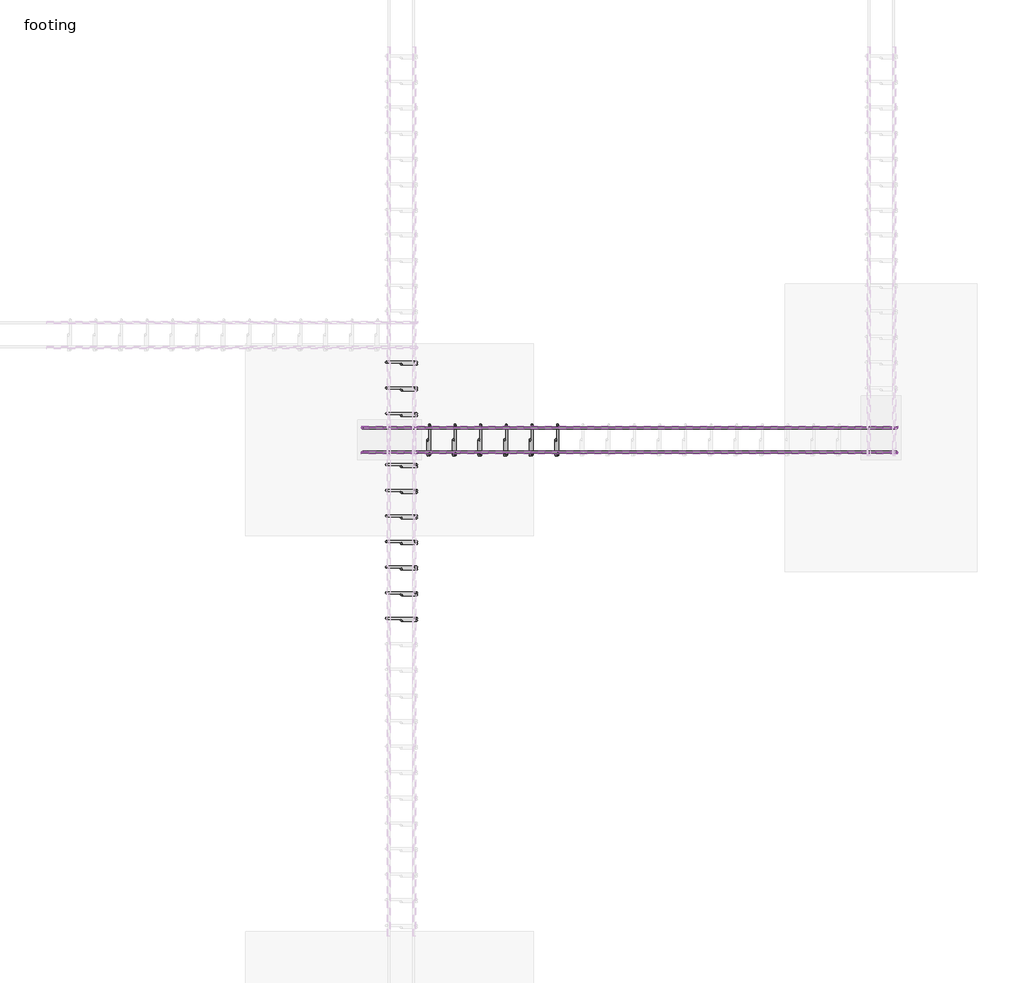
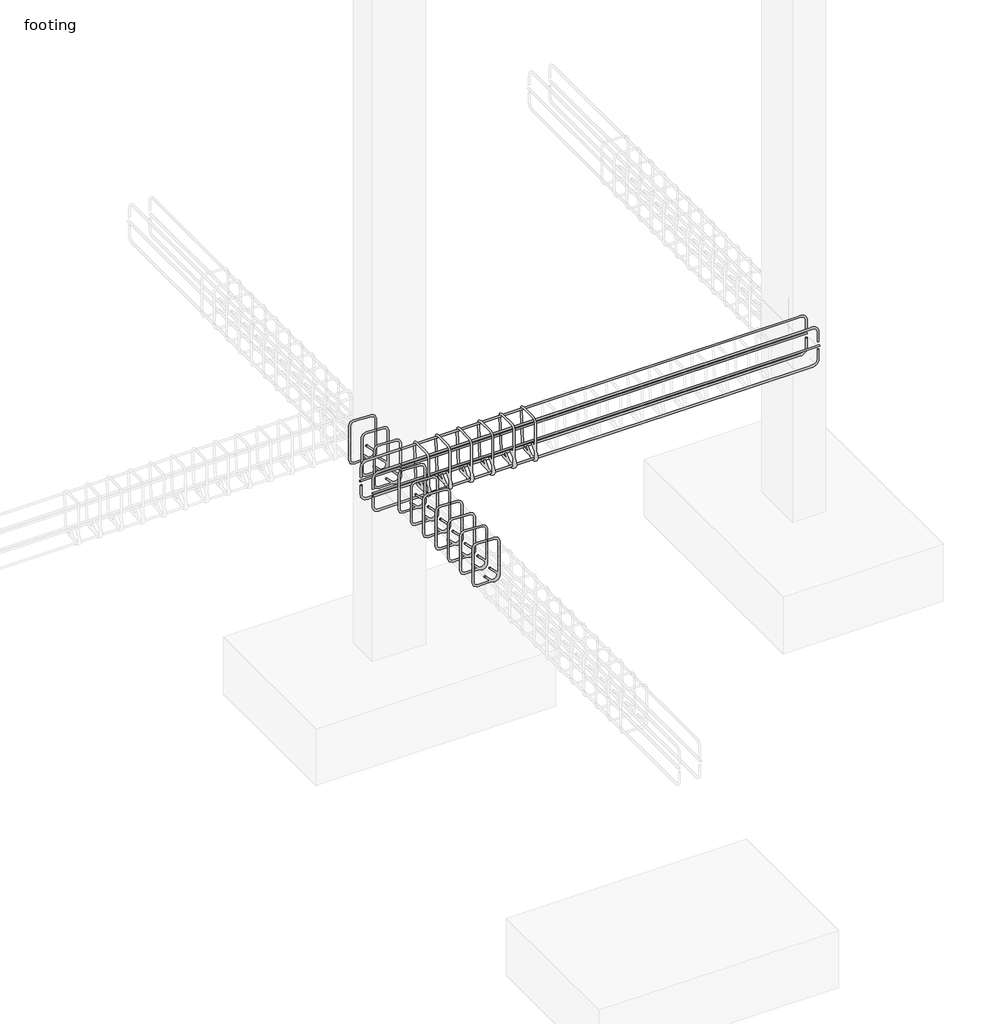
# One storey, part 10 of 21: 22 reinforcing bars.
"""IFC4 building model written with IfcOpenShell, lengths in millimetres."""

from ifc_helpers import new_model, si_unit, point, frame, origin, place, context, project, spatial, polyline, circle_curve, trimmed, segment, composite_curve, element, save
from ifc_brep_helpers import swept_disk

model = new_model("IFC4")

# Units and contexts
model_context = context("Model", 3, world=origin())
ifc_project = project(units=[si_unit("LENGTHUNIT", "METRE", prefix="MILLI")], contexts=[model_context])

# Site, building, storey
site = spatial("IfcSite", under=ifc_project)
building = spatial("IfcBuilding", under=site)
storey = spatial("IfcBuildingStorey", under=building, Name="footing", Elevation=-1524.0)

# Reinforcing bars
placement = place(None, origin())
element("IfcReinforcingBar", 1, at=placement, inside=storey, context=model_context, shape_type="SolidModel", body=[
    swept_disk(composite_curve([segment(polyline([(-7699.7883428, 3451.1387132, -310.8825168), (-7699.7883428, 3396.2737147, -365.7475153)]), True, "CONTINUOUS"), segment(trimmed(circle_curve(frame((-7699.7883428, 3373.8230744, -343.296875), z_axis=(-1.0, 0.0, 0.0), x_axis=(0.0, 22.450640299999577, -22.450640299999975)), 31.75), [point((-7699.7883428, 3396.2737147, -365.7475153))], [point((-7699.7883428, 3342.0730744, -343.296875))], True, "CARTESIAN"), True, "CONTINUOUS"), segment(polyline([(-7699.7883428, 3342.0730744, -343.296875), (-7699.7883428, 3342.0730744, -63.103125)]), True, "CONTINUOUS"), segment(trimmed(circle_curve(frame((-7699.7883428, 3373.8230744, -63.103125), z_axis=(-1.0, 0.0, 0.0), x_axis=(0.0, -31.75, 0.0)), 31.75), [point((-7699.7883428, 3342.0730744, -63.103125))], [point((-7699.7883428, 3373.8230744, -31.353125))], True, "CARTESIAN"), True, "CONTINUOUS"), segment(polyline([(-7699.7883428, 3373.8230744, -31.353125), (-7699.7883428, 3501.6168244, -31.353125)]), True, "CONTINUOUS"), segment(trimmed(circle_curve(frame((-7698.6159328, 3501.6168244, -63.0814712), z_axis=(-0.9993179916193466, 0.0, -0.03692629992126919), x_axis=(-1.1724099999992177, 0.0, 31.728346200000004)), 31.75), [point((-7699.7883428, 3501.6168244, -31.353125))], [point((-7698.6159328, 3533.3668244, -63.0814712))], True, "CARTESIAN"), True, "CONTINUOUS"), segment(polyline([(-7698.6159328, 3533.3668244, -63.0814712), (-7688.2607528, 3533.3668244, -343.3185288)]), True, "CONTINUOUS"), segment(trimmed(circle_curve(frame((-7688.2607528, 3501.6168244, -343.3185288), z_axis=(-0.9993179916193466, 0.0, -0.03692629992126919), x_axis=(0.0, 31.75, 0.0)), 31.75), [point((-7688.2607528, 3533.3668244, -343.3185288))], [point((-7687.0883428, 3501.6168244, -375.046875))], True, "CARTESIAN"), True, "CONTINUOUS"), segment(polyline([(-7687.0883428, 3501.6168244, -375.046875), (-7687.0883428, 3373.8230744, -375.046875)]), True, "CONTINUOUS"), segment(trimmed(circle_curve(frame((-7687.0883428, 3373.8230744, -343.296875), z_axis=(-1.0, 0.0, 0.0), x_axis=(0.0, 0.0, -31.75)), 31.75), [point((-7687.0883428, 3373.8230744, -375.046875))], [point((-7687.0883428, 3351.3724341, -320.8462347))], True, "CARTESIAN"), True, "CONTINUOUS"), segment(polyline([(-7687.0883428, 3351.3724341, -320.8462347), (-7687.0883428, 3406.2374326, -265.9812362)]), True, "CONTINUOUS")], self_intersect=False), 6.35),
])
element("IfcReinforcingBar", 2, at=placement, inside=storey, context=model_context, shape_type="SolidModel", body=[
    swept_disk(composite_curve([segment(polyline([(-4722.5521673, 3515.0872086, -236.1172592), (-4722.5521673, 3515.0872086, -312.3172592)]), True, "CONTINUOUS"), segment(trimmed(circle_curve(frame((-4767.0021673, 3515.0872086, -312.3172592), z_axis=(0.0, 1.0, -2.1166279873208456e-12), x_axis=(44.44999999999982, 0.0, 0.0)), 44.45), [point((-4722.5521673, 3515.0872086, -312.3172592))], [point((-4767.0021673, 3515.0872086, -356.7672592))], True, "CARTESIAN"), True, "CONTINUOUS"), segment(polyline([(-4767.0021673, 3515.0872086, -356.7672592), (-8069.7959173, 3515.0872086, -356.7672592)]), True, "CONTINUOUS"), segment(trimmed(circle_curve(frame((-8069.7959173, 3515.0872086, -312.3172592), z_axis=(0.0, 1.0, -2.1166279873208456e-12), x_axis=(0.0, 0.0, -44.44999999999999)), 44.45), [point((-8069.7959173, 3515.0872086, -356.7672592))], [point((-8114.2459173, 3515.0872086, -312.3172592))], True, "CARTESIAN"), True, "CONTINUOUS"), segment(polyline([(-8114.2459173, 3515.0872086, -312.3172592), (-8114.2459173, 3515.0872086, -236.1172592)]), True, "CONTINUOUS")], self_intersect=False), 6.35),
])
element("IfcReinforcingBar", 3, at=placement, inside=storey, context=model_context, shape_type="SolidModel", body=[
    swept_disk(composite_curve([segment(polyline([(-4722.5521673, 3360.3526902, -170.2827408), (-4722.5521673, 3360.3526902, -94.0827408)]), True, "CONTINUOUS"), segment(trimmed(circle_curve(frame((-4767.0021673, 3360.3526902, -94.0827408), z_axis=(0.0, -1.0, 0.0), x_axis=(44.44999999999982, 0.0, 0.0)), 44.45), [point((-4722.5521673, 3360.3526902, -94.0827408))], [point((-4767.0021673, 3360.3526902, -49.6327408))], True, "CARTESIAN"), True, "CONTINUOUS"), segment(polyline([(-4767.0021673, 3360.3526902, -49.6327408), (-8069.7959173, 3360.3526902, -49.6327408)]), True, "CONTINUOUS"), segment(trimmed(circle_curve(frame((-8069.7959173, 3360.3526902, -94.0827408), z_axis=(0.0, -1.0, 0.0), x_axis=(0.0, 0.0, 44.449999999999996)), 44.45), [point((-8069.7959173, 3360.3526902, -49.6327408))], [point((-8114.2459173, 3360.3526902, -94.0827408))], True, "CARTESIAN"), True, "CONTINUOUS"), segment(polyline([(-8114.2459173, 3360.3526902, -94.0827408), (-8114.2459173, 3360.3526902, -170.2827408)]), True, "CONTINUOUS")], self_intersect=False), 6.35),
])
element("IfcReinforcingBar", 4, at=placement, inside=storey, context=model_context, shape_type="SolidModel", body=[
    swept_disk(composite_curve([segment(polyline([(-4722.5521673, 3360.3526902, -236.1172592), (-4722.5521673, 3360.3526902, -312.3172592)]), True, "CONTINUOUS"), segment(trimmed(circle_curve(frame((-4767.0021673, 3360.3526902, -312.3172592), z_axis=(0.0, 1.0, 2.1166279873208456e-12), x_axis=(44.44999999999982, 0.0, 0.0)), 44.45), [point((-4722.5521673, 3360.3526902, -312.3172592))], [point((-4767.0021673, 3360.3526902, -356.7672592))], True, "CARTESIAN"), True, "CONTINUOUS"), segment(polyline([(-4767.0021673, 3360.3526902, -356.7672592), (-8069.7959173, 3360.3526902, -356.7672592)]), True, "CONTINUOUS"), segment(trimmed(circle_curve(frame((-8069.7959173, 3360.3526902, -312.3172592), z_axis=(0.0, 1.0, 2.1166279873208456e-12), x_axis=(0.0, 0.0, -44.44999999999999)), 44.45), [point((-8069.7959173, 3360.3526902, -356.7672592))], [point((-8114.2459173, 3360.3526902, -312.3172592))], True, "CARTESIAN"), True, "CONTINUOUS"), segment(polyline([(-8114.2459173, 3360.3526902, -312.3172592), (-8114.2459173, 3360.3526902, -236.1172592)]), True, "CONTINUOUS")], self_intersect=False), 6.35),
])
element("IfcReinforcingBar", 5, at=placement, inside=storey, context=model_context, shape_type="SolidModel", body=[
    swept_disk(composite_curve([segment(polyline([(-4722.5521673, 3515.0872086, -170.2827408), (-4722.5521673, 3515.0872086, -94.0827408)]), True, "CONTINUOUS"), segment(trimmed(circle_curve(frame((-4767.0021673, 3515.0872086, -94.0827408), z_axis=(0.0, -1.0, 0.0), x_axis=(44.44999999999982, 0.0, 0.0)), 44.45), [point((-4722.5521673, 3515.0872086, -94.0827408))], [point((-4767.0021673, 3515.0872086, -49.6327408))], True, "CARTESIAN"), True, "CONTINUOUS"), segment(polyline([(-4767.0021673, 3515.0872086, -49.6327408), (-8069.7959173, 3515.0872086, -49.6327408)]), True, "CONTINUOUS"), segment(trimmed(circle_curve(frame((-8069.7959173, 3515.0872086, -94.0827408), z_axis=(0.0, -1.0, 0.0), x_axis=(0.0, 0.0, 44.449999999999996)), 44.45), [point((-8069.7959173, 3515.0872086, -49.6327408))], [point((-8114.2459173, 3515.0872086, -94.0827408))], True, "CARTESIAN"), True, "CONTINUOUS"), segment(polyline([(-8114.2459173, 3515.0872086, -94.0827408), (-8114.2459173, 3515.0872086, -170.2827408)]), True, "CONTINUOUS")], self_intersect=False), 6.35),
])
element("IfcReinforcingBar", 6, at=placement, inside=storey, context=model_context, shape_type="SolidModel", body=[
    swept_disk(composite_curve([segment(polyline([(-4716.2021673, 3520.6668244, -203.2), (-8120.5959173, 3520.6668244, -203.2)]), True, "CONTINUOUS")], self_intersect=False), 6.35),
])
element("IfcReinforcingBar", 7, at=placement, inside=storey, context=model_context, shape_type="SolidModel", body=[
    swept_disk(composite_curve([segment(polyline([(-4716.2021673, 3354.7730744, -203.2), (-8120.5959173, 3354.7730744, -203.2)]), True, "CONTINUOUS")], self_intersect=False), 6.35),
])
element("IfcReinforcingBar", 8, at=placement, inside=storey, context=model_context, shape_type="SolidModel", body=[
    swept_disk(composite_curve([segment(polyline([(-7537.0883428, 3451.1387132, -310.8825168), (-7537.0883428, 3396.2737147, -365.7475153)]), True, "CONTINUOUS"), segment(trimmed(circle_curve(frame((-7537.0883428, 3373.8230744, -343.296875), z_axis=(-1.0, 0.0, 0.0), x_axis=(0.0, 22.450640299999577, -22.450640299999975)), 31.75), [point((-7537.0883428, 3396.2737147, -365.7475153))], [point((-7537.0883428, 3342.0730744, -343.296875))], True, "CARTESIAN"), True, "CONTINUOUS"), segment(polyline([(-7537.0883428, 3342.0730744, -343.296875), (-7537.0883428, 3342.0730744, -63.103125)]), True, "CONTINUOUS"), segment(trimmed(circle_curve(frame((-7537.0883428, 3373.8230744, -63.103125), z_axis=(-1.0, 0.0, 0.0), x_axis=(0.0, -31.75, 0.0)), 31.75), [point((-7537.0883428, 3342.0730744, -63.103125))], [point((-7537.0883428, 3373.8230744, -31.353125))], True, "CARTESIAN"), True, "CONTINUOUS"), segment(polyline([(-7537.0883428, 3373.8230744, -31.353125), (-7537.0883428, 3501.6168244, -31.353125)]), True, "CONTINUOUS"), segment(trimmed(circle_curve(frame((-7535.9159328, 3501.6168244, -63.0814712), z_axis=(-0.9993179916193466, 0.0, -0.03692629992126919), x_axis=(-1.1724100000001272, 0.0, 31.728346200000004)), 31.75), [point((-7537.0883428, 3501.6168244, -31.353125))], [point((-7535.9159328, 3533.3668244, -63.0814712))], True, "CARTESIAN"), True, "CONTINUOUS"), segment(polyline([(-7535.9159328, 3533.3668244, -63.0814712), (-7525.5607528, 3533.3668244, -343.3185288)]), True, "CONTINUOUS"), segment(trimmed(circle_curve(frame((-7525.5607528, 3501.6168244, -343.3185288), z_axis=(-0.9993179916193466, 0.0, -0.03692629992126919), x_axis=(0.0, 31.75, 0.0)), 31.75), [point((-7525.5607528, 3533.3668244, -343.3185288))], [point((-7524.3883428, 3501.6168244, -375.046875))], True, "CARTESIAN"), True, "CONTINUOUS"), segment(polyline([(-7524.3883428, 3501.6168244, -375.046875), (-7524.3883428, 3373.8230744, -375.046875)]), True, "CONTINUOUS"), segment(trimmed(circle_curve(frame((-7524.3883428, 3373.8230744, -343.296875), z_axis=(-1.0, 0.0, 0.0), x_axis=(0.0, 0.0, -31.75)), 31.75), [point((-7524.3883428, 3373.8230744, -375.046875))], [point((-7524.3883428, 3351.3724341, -320.8462347))], True, "CARTESIAN"), True, "CONTINUOUS"), segment(polyline([(-7524.3883428, 3351.3724341, -320.8462347), (-7524.3883428, 3406.2374326, -265.9812362)]), True, "CONTINUOUS")], self_intersect=False), 6.35),
])
element("IfcReinforcingBar", 9, at=placement, inside=storey, context=model_context, shape_type="SolidModel", body=[
    swept_disk(composite_curve([segment(polyline([(-7374.3883428, 3451.1387132, -310.8825168), (-7374.3883428, 3396.2737147, -365.7475153)]), True, "CONTINUOUS"), segment(trimmed(circle_curve(frame((-7374.3883428, 3373.8230744, -343.296875), z_axis=(-1.0, 0.0, 0.0), x_axis=(0.0, 22.450640299999577, -22.450640299999975)), 31.75), [point((-7374.3883428, 3396.2737147, -365.7475153))], [point((-7374.3883428, 3342.0730744, -343.296875))], True, "CARTESIAN"), True, "CONTINUOUS"), segment(polyline([(-7374.3883428, 3342.0730744, -343.296875), (-7374.3883428, 3342.0730744, -63.103125)]), True, "CONTINUOUS"), segment(trimmed(circle_curve(frame((-7374.3883428, 3373.8230744, -63.103125), z_axis=(-1.0, 0.0, 0.0), x_axis=(0.0, -31.75, 0.0)), 31.75), [point((-7374.3883428, 3342.0730744, -63.103125))], [point((-7374.3883428, 3373.8230744, -31.353125))], True, "CARTESIAN"), True, "CONTINUOUS"), segment(polyline([(-7374.3883428, 3373.8230744, -31.353125), (-7374.3883428, 3501.6168244, -31.353125)]), True, "CONTINUOUS"), segment(trimmed(circle_curve(frame((-7373.2159328, 3501.6168244, -63.0814712), z_axis=(-0.9993179916193466, 0.0, -0.03692629992126919), x_axis=(-1.1724100000001272, 0.0, 31.728346200000004)), 31.75), [point((-7374.3883428, 3501.6168244, -31.353125))], [point((-7373.2159328, 3533.3668244, -63.0814712))], True, "CARTESIAN"), True, "CONTINUOUS"), segment(polyline([(-7373.2159328, 3533.3668244, -63.0814712), (-7362.8607528, 3533.3668244, -343.3185288)]), True, "CONTINUOUS"), segment(trimmed(circle_curve(frame((-7362.8607528, 3501.6168244, -343.3185288), z_axis=(-0.9993179916193466, 0.0, -0.03692629992126919), x_axis=(0.0, 31.75, 0.0)), 31.75), [point((-7362.8607528, 3533.3668244, -343.3185288))], [point((-7361.6883428, 3501.6168244, -375.046875))], True, "CARTESIAN"), True, "CONTINUOUS"), segment(polyline([(-7361.6883428, 3501.6168244, -375.046875), (-7361.6883428, 3373.8230744, -375.046875)]), True, "CONTINUOUS"), segment(trimmed(circle_curve(frame((-7361.6883428, 3373.8230744, -343.296875), z_axis=(-1.0, 0.0, 0.0), x_axis=(0.0, 0.0, -31.75)), 31.75), [point((-7361.6883428, 3373.8230744, -375.046875))], [point((-7361.6883428, 3351.3724341, -320.8462347))], True, "CARTESIAN"), True, "CONTINUOUS"), segment(polyline([(-7361.6883428, 3351.3724341, -320.8462347), (-7361.6883428, 3406.2374326, -265.9812362)]), True, "CONTINUOUS")], self_intersect=False), 6.35),
])
element("IfcReinforcingBar", 10, at=placement, inside=storey, context=model_context, shape_type="SolidModel", body=[
    swept_disk(composite_curve([segment(polyline([(-7211.6883428, 3451.1387132, -310.8825168), (-7211.6883428, 3396.2737147, -365.7475153)]), True, "CONTINUOUS"), segment(trimmed(circle_curve(frame((-7211.6883428, 3373.8230744, -343.296875), z_axis=(-1.0, 0.0, 0.0), x_axis=(0.0, 22.450640299999577, -22.450640299999975)), 31.75), [point((-7211.6883428, 3396.2737147, -365.7475153))], [point((-7211.6883428, 3342.0730744, -343.296875))], True, "CARTESIAN"), True, "CONTINUOUS"), segment(polyline([(-7211.6883428, 3342.0730744, -343.296875), (-7211.6883428, 3342.0730744, -63.103125)]), True, "CONTINUOUS"), segment(trimmed(circle_curve(frame((-7211.6883428, 3373.8230744, -63.103125), z_axis=(-1.0, 0.0, 0.0), x_axis=(0.0, -31.75, 0.0)), 31.75), [point((-7211.6883428, 3342.0730744, -63.103125))], [point((-7211.6883428, 3373.8230744, -31.353125))], True, "CARTESIAN"), True, "CONTINUOUS"), segment(polyline([(-7211.6883428, 3373.8230744, -31.353125), (-7211.6883428, 3501.6168244, -31.353125)]), True, "CONTINUOUS"), segment(trimmed(circle_curve(frame((-7210.5159328, 3501.6168244, -63.0814712), z_axis=(-0.9993179916193466, 0.0, -0.03692629992126919), x_axis=(-1.1724100000001272, 0.0, 31.728346200000004)), 31.75), [point((-7211.6883428, 3501.6168244, -31.353125))], [point((-7210.5159328, 3533.3668244, -63.0814712))], True, "CARTESIAN"), True, "CONTINUOUS"), segment(polyline([(-7210.5159328, 3533.3668244, -63.0814712), (-7200.1607528, 3533.3668244, -343.3185288)]), True, "CONTINUOUS"), segment(trimmed(circle_curve(frame((-7200.1607528, 3501.6168244, -343.3185288), z_axis=(-0.9993179916193466, 0.0, -0.03692629992126919), x_axis=(0.0, 31.75, 0.0)), 31.75), [point((-7200.1607528, 3533.3668244, -343.3185288))], [point((-7198.9883428, 3501.6168244, -375.046875))], True, "CARTESIAN"), True, "CONTINUOUS"), segment(polyline([(-7198.9883428, 3501.6168244, -375.046875), (-7198.9883428, 3373.8230744, -375.046875)]), True, "CONTINUOUS"), segment(trimmed(circle_curve(frame((-7198.9883428, 3373.8230744, -343.296875), z_axis=(-1.0, 0.0, 0.0), x_axis=(0.0, 0.0, -31.75)), 31.75), [point((-7198.9883428, 3373.8230744, -375.046875))], [point((-7198.9883428, 3351.3724341, -320.8462347))], True, "CARTESIAN"), True, "CONTINUOUS"), segment(polyline([(-7198.9883428, 3351.3724341, -320.8462347), (-7198.9883428, 3406.2374326, -265.9812362)]), True, "CONTINUOUS")], self_intersect=False), 6.35),
])
element("IfcReinforcingBar", 11, at=placement, inside=storey, context=model_context, shape_type="SolidModel", body=[
    swept_disk(composite_curve([segment(polyline([(-7048.9883428, 3451.1387132, -310.8825168), (-7048.9883428, 3396.2737147, -365.7475153)]), True, "CONTINUOUS"), segment(trimmed(circle_curve(frame((-7048.9883428, 3373.8230744, -343.296875), z_axis=(-1.0, 0.0, 0.0), x_axis=(0.0, 22.450640299999577, -22.450640299999975)), 31.75), [point((-7048.9883428, 3396.2737147, -365.7475153))], [point((-7048.9883428, 3342.0730744, -343.296875))], True, "CARTESIAN"), True, "CONTINUOUS"), segment(polyline([(-7048.9883428, 3342.0730744, -343.296875), (-7048.9883428, 3342.0730744, -63.103125)]), True, "CONTINUOUS"), segment(trimmed(circle_curve(frame((-7048.9883428, 3373.8230744, -63.103125), z_axis=(-1.0, 0.0, 0.0), x_axis=(0.0, -31.75, 0.0)), 31.75), [point((-7048.9883428, 3342.0730744, -63.103125))], [point((-7048.9883428, 3373.8230744, -31.353125))], True, "CARTESIAN"), True, "CONTINUOUS"), segment(polyline([(-7048.9883428, 3373.8230744, -31.353125), (-7048.9883428, 3501.6168244, -31.353125)]), True, "CONTINUOUS"), segment(trimmed(circle_curve(frame((-7047.8159328, 3501.6168244, -63.0814712), z_axis=(-0.9993179916193466, 0.0, -0.03692629992126919), x_axis=(-1.1724100000001272, 0.0, 31.728346200000004)), 31.75), [point((-7048.9883428, 3501.6168244, -31.353125))], [point((-7047.8159328, 3533.3668244, -63.0814712))], True, "CARTESIAN"), True, "CONTINUOUS"), segment(polyline([(-7047.8159328, 3533.3668244, -63.0814712), (-7037.4607528, 3533.3668244, -343.3185288)]), True, "CONTINUOUS"), segment(trimmed(circle_curve(frame((-7037.4607528, 3501.6168244, -343.3185288), z_axis=(-0.9993179916193466, 0.0, -0.03692629992126919), x_axis=(0.0, 31.75, 0.0)), 31.75), [point((-7037.4607528, 3533.3668244, -343.3185288))], [point((-7036.2883428, 3501.6168244, -375.046875))], True, "CARTESIAN"), True, "CONTINUOUS"), segment(polyline([(-7036.2883428, 3501.6168244, -375.046875), (-7036.2883428, 3373.8230744, -375.046875)]), True, "CONTINUOUS"), segment(trimmed(circle_curve(frame((-7036.2883428, 3373.8230744, -343.296875), z_axis=(-1.0, 0.0, 0.0), x_axis=(0.0, 0.0, -31.75)), 31.75), [point((-7036.2883428, 3373.8230744, -375.046875))], [point((-7036.2883428, 3351.3724341, -320.8462347))], True, "CARTESIAN"), True, "CONTINUOUS"), segment(polyline([(-7036.2883428, 3351.3724341, -320.8462347), (-7036.2883428, 3406.2374326, -265.9812362)]), True, "CONTINUOUS")], self_intersect=False), 6.35),
])
element("IfcReinforcingBar", 12, at=placement, inside=storey, context=model_context, shape_type="SolidModel", body=[
    swept_disk(composite_curve([segment(polyline([(-6886.2883428, 3451.1387132, -310.8825168), (-6886.2883428, 3396.2737147, -365.7475153)]), True, "CONTINUOUS"), segment(trimmed(circle_curve(frame((-6886.2883428, 3373.8230744, -343.296875), z_axis=(-1.0, 0.0, 0.0), x_axis=(0.0, 22.450640299999577, -22.450640299999975)), 31.75), [point((-6886.2883428, 3396.2737147, -365.7475153))], [point((-6886.2883428, 3342.0730744, -343.296875))], True, "CARTESIAN"), True, "CONTINUOUS"), segment(polyline([(-6886.2883428, 3342.0730744, -343.296875), (-6886.2883428, 3342.0730744, -63.103125)]), True, "CONTINUOUS"), segment(trimmed(circle_curve(frame((-6886.2883428, 3373.8230744, -63.103125), z_axis=(-1.0, 0.0, 0.0), x_axis=(0.0, -31.75, 0.0)), 31.75), [point((-6886.2883428, 3342.0730744, -63.103125))], [point((-6886.2883428, 3373.8230744, -31.353125))], True, "CARTESIAN"), True, "CONTINUOUS"), segment(polyline([(-6886.2883428, 3373.8230744, -31.353125), (-6886.2883428, 3501.6168244, -31.353125)]), True, "CONTINUOUS"), segment(trimmed(circle_curve(frame((-6885.1159328, 3501.6168244, -63.0814712), z_axis=(-0.9993179916193466, 0.0, -0.03692629992126919), x_axis=(-1.1724099999992177, 0.0, 31.728346200000004)), 31.75), [point((-6886.2883428, 3501.6168244, -31.353125))], [point((-6885.1159328, 3533.3668244, -63.0814712))], True, "CARTESIAN"), True, "CONTINUOUS"), segment(polyline([(-6885.1159328, 3533.3668244, -63.0814712), (-6874.7607528, 3533.3668244, -343.3185288)]), True, "CONTINUOUS"), segment(trimmed(circle_curve(frame((-6874.7607528, 3501.6168244, -343.3185288), z_axis=(-0.9993179916193466, 0.0, -0.03692629992126919), x_axis=(0.0, 31.75, 0.0)), 31.75), [point((-6874.7607528, 3533.3668244, -343.3185288))], [point((-6873.5883428, 3501.6168244, -375.046875))], True, "CARTESIAN"), True, "CONTINUOUS"), segment(polyline([(-6873.5883428, 3501.6168244, -375.046875), (-6873.5883428, 3373.8230744, -375.046875)]), True, "CONTINUOUS"), segment(trimmed(circle_curve(frame((-6873.5883428, 3373.8230744, -343.296875), z_axis=(-1.0, 0.0, 0.0), x_axis=(0.0, 0.0, -31.75)), 31.75), [point((-6873.5883428, 3373.8230744, -375.046875))], [point((-6873.5883428, 3351.3724341, -320.8462347))], True, "CARTESIAN"), True, "CONTINUOUS"), segment(polyline([(-6873.5883428, 3351.3724341, -320.8462347), (-6873.5883428, 3406.2374326, -265.9812362)]), True, "CONTINUOUS")], self_intersect=False), 6.35),
])
element("IfcReinforcingBar", 13, at=placement, inside=storey, context=model_context, shape_type="SolidModel", body=[
    swept_disk(composite_curve([segment(polyline([(-7834.7165254, 2304.6956073, -265.9812362), (-7779.851527, 2304.6956073, -320.8462347)]), True, "CONTINUOUS"), segment(trimmed(circle_curve(frame((-7802.3021673, 2304.6956073, -343.296875), z_axis=(0.0, 1.0, 0.0), x_axis=(22.450640300000487, 0.0, 22.450640299999975)), 31.75), [point((-7779.851527, 2304.6956073, -320.8462347))], [point((-7802.3021673, 2304.6956073, -375.046875))], True, "CARTESIAN"), True, "CONTINUOUS"), segment(polyline([(-7802.3021673, 2304.6956073, -375.046875), (-7930.0959173, 2304.6956073, -375.046875)]), True, "CONTINUOUS"), segment(trimmed(circle_curve(frame((-7930.0959173, 2304.6956073, -343.296875), z_axis=(0.0, 1.0, 0.0), x_axis=(0.0, 0.0, -31.75)), 31.75), [point((-7930.0959173, 2304.6956073, -375.046875))], [point((-7961.8459173, 2304.6956073, -343.296875))], True, "CARTESIAN"), True, "CONTINUOUS"), segment(polyline([(-7961.8459173, 2304.6956073, -343.296875), (-7961.8459173, 2304.6956073, -63.103125)]), True, "CONTINUOUS"), segment(trimmed(circle_curve(frame((-7930.165658, 2302.5923536, -63.103125), z_axis=(0.0662442117686417, 0.9978034397651431, 0.0), x_axis=(-31.680259300000216, 2.1032537000000957, 0.0)), 31.75), [point((-7961.8459173, 2304.6956073, -63.103125))], [point((-7930.165658, 2302.5923536, -31.353125))], True, "CARTESIAN"), True, "CONTINUOUS"), segment(polyline([(-7930.165658, 2302.5923536, -31.353125), (-7802.2324265, 2294.098861, -31.353125)]), True, "CONTINUOUS"), segment(trimmed(circle_curve(frame((-7802.2324265, 2294.098861, -63.103125), z_axis=(0.06624421176864169, 0.997803439765143, 0.0), x_axis=(0.0, 0.0, 31.75)), 31.75), [point((-7802.2324265, 2294.098861, -31.353125))], [point((-7770.5521673, 2291.9956073, -63.103125))], True, "CARTESIAN"), True, "CONTINUOUS"), segment(polyline([(-7770.5521673, 2291.9956073, -63.103125), (-7770.5521673, 2291.9956073, -343.296875)]), True, "CONTINUOUS"), segment(trimmed(circle_curve(frame((-7802.3021673, 2291.9956073, -343.296875), z_axis=(0.0, 1.0, 0.0), x_axis=(31.75, 0.0, 0.0)), 31.75), [point((-7770.5521673, 2291.9956073, -343.296875))], [point((-7824.7528076, 2291.9956073, -365.7475153))], True, "CARTESIAN"), True, "CONTINUOUS"), segment(polyline([(-7824.7528076, 2291.9956073, -365.7475153), (-7879.617806, 2291.9956073, -310.8825168)]), True, "CONTINUOUS")], self_intersect=False), 6.35),
])
element("IfcReinforcingBar", 14, at=placement, inside=storey, context=model_context, shape_type="SolidModel", body=[
    swept_disk(composite_curve([segment(polyline([(-7834.7165254, 2467.3956073, -265.9812362), (-7779.851527, 2467.3956073, -320.8462347)]), True, "CONTINUOUS"), segment(trimmed(circle_curve(frame((-7802.3021673, 2467.3956073, -343.296875), z_axis=(0.0, 1.0, 0.0), x_axis=(22.450640300000487, 0.0, 22.450640299999975)), 31.75), [point((-7779.851527, 2467.3956073, -320.8462347))], [point((-7802.3021673, 2467.3956073, -375.046875))], True, "CARTESIAN"), True, "CONTINUOUS"), segment(polyline([(-7802.3021673, 2467.3956073, -375.046875), (-7930.0959173, 2467.3956073, -375.046875)]), True, "CONTINUOUS"), segment(trimmed(circle_curve(frame((-7930.0959173, 2467.3956073, -343.296875), z_axis=(0.0, 1.0, 0.0), x_axis=(0.0, 0.0, -31.75)), 31.75), [point((-7930.0959173, 2467.3956073, -375.046875))], [point((-7961.8459173, 2467.3956073, -343.296875))], True, "CARTESIAN"), True, "CONTINUOUS"), segment(polyline([(-7961.8459173, 2467.3956073, -343.296875), (-7961.8459173, 2467.3956073, -63.103125)]), True, "CONTINUOUS"), segment(trimmed(circle_curve(frame((-7930.165658, 2465.2923536, -63.103125), z_axis=(0.0662442117686417, 0.9978034397651431, 0.0), x_axis=(-31.680259300000216, 2.1032537000000957, 0.0)), 31.75), [point((-7961.8459173, 2467.3956073, -63.103125))], [point((-7930.165658, 2465.2923536, -31.353125))], True, "CARTESIAN"), True, "CONTINUOUS"), segment(polyline([(-7930.165658, 2465.2923536, -31.353125), (-7802.2324265, 2456.798861, -31.353125)]), True, "CONTINUOUS"), segment(trimmed(circle_curve(frame((-7802.2324265, 2456.798861, -63.103125), z_axis=(0.06624421176864169, 0.997803439765143, 0.0), x_axis=(0.0, 0.0, 31.75)), 31.75), [point((-7802.2324265, 2456.798861, -31.353125))], [point((-7770.5521673, 2454.6956073, -63.103125))], True, "CARTESIAN"), True, "CONTINUOUS"), segment(polyline([(-7770.5521673, 2454.6956073, -63.103125), (-7770.5521673, 2454.6956073, -343.296875)]), True, "CONTINUOUS"), segment(trimmed(circle_curve(frame((-7802.3021673, 2454.6956073, -343.296875), z_axis=(0.0, 1.0, 0.0), x_axis=(31.75, 0.0, 0.0)), 31.75), [point((-7770.5521673, 2454.6956073, -343.296875))], [point((-7824.7528076, 2454.6956073, -365.7475153))], True, "CARTESIAN"), True, "CONTINUOUS"), segment(polyline([(-7824.7528076, 2454.6956073, -365.7475153), (-7879.617806, 2454.6956073, -310.8825168)]), True, "CONTINUOUS")], self_intersect=False), 6.35),
])
element("IfcReinforcingBar", 15, at=placement, inside=storey, context=model_context, shape_type="SolidModel", body=[
    swept_disk(composite_curve([segment(polyline([(-7834.7165254, 2630.0956073, -265.9812362), (-7779.851527, 2630.0956073, -320.8462347)]), True, "CONTINUOUS"), segment(trimmed(circle_curve(frame((-7802.3021673, 2630.0956073, -343.296875), z_axis=(0.0, 1.0, 0.0), x_axis=(22.450640300000487, 0.0, 22.450640299999975)), 31.75), [point((-7779.851527, 2630.0956073, -320.8462347))], [point((-7802.3021673, 2630.0956073, -375.046875))], True, "CARTESIAN"), True, "CONTINUOUS"), segment(polyline([(-7802.3021673, 2630.0956073, -375.046875), (-7930.0959173, 2630.0956073, -375.046875)]), True, "CONTINUOUS"), segment(trimmed(circle_curve(frame((-7930.0959173, 2630.0956073, -343.296875), z_axis=(0.0, 1.0, 0.0), x_axis=(0.0, 0.0, -31.75)), 31.75), [point((-7930.0959173, 2630.0956073, -375.046875))], [point((-7961.8459173, 2630.0956073, -343.296875))], True, "CARTESIAN"), True, "CONTINUOUS"), segment(polyline([(-7961.8459173, 2630.0956073, -343.296875), (-7961.8459173, 2630.0956073, -63.103125)]), True, "CONTINUOUS"), segment(trimmed(circle_curve(frame((-7930.165658, 2627.9923536, -63.103125), z_axis=(0.0662442117686417, 0.9978034397651431, 0.0), x_axis=(-31.680259300000216, 2.1032537000000957, 0.0)), 31.75), [point((-7961.8459173, 2630.0956073, -63.103125))], [point((-7930.165658, 2627.9923536, -31.353125))], True, "CARTESIAN"), True, "CONTINUOUS"), segment(polyline([(-7930.165658, 2627.9923536, -31.353125), (-7802.2324265, 2619.498861, -31.353125)]), True, "CONTINUOUS"), segment(trimmed(circle_curve(frame((-7802.2324265, 2619.498861, -63.103125), z_axis=(0.06624421176864169, 0.997803439765143, 0.0), x_axis=(0.0, 0.0, 31.75)), 31.75), [point((-7802.2324265, 2619.498861, -31.353125))], [point((-7770.5521673, 2617.3956073, -63.103125))], True, "CARTESIAN"), True, "CONTINUOUS"), segment(polyline([(-7770.5521673, 2617.3956073, -63.103125), (-7770.5521673, 2617.3956073, -343.296875)]), True, "CONTINUOUS"), segment(trimmed(circle_curve(frame((-7802.3021673, 2617.3956073, -343.296875), z_axis=(0.0, 1.0, 0.0), x_axis=(31.75, 0.0, 0.0)), 31.75), [point((-7770.5521673, 2617.3956073, -343.296875))], [point((-7824.7528076, 2617.3956073, -365.7475153))], True, "CARTESIAN"), True, "CONTINUOUS"), segment(polyline([(-7824.7528076, 2617.3956073, -365.7475153), (-7879.617806, 2617.3956073, -310.8825168)]), True, "CONTINUOUS")], self_intersect=False), 6.35),
])
element("IfcReinforcingBar", 16, at=placement, inside=storey, context=model_context, shape_type="SolidModel", body=[
    swept_disk(composite_curve([segment(polyline([(-7834.7165254, 2792.7956073, -265.9812362), (-7779.851527, 2792.7956073, -320.8462347)]), True, "CONTINUOUS"), segment(trimmed(circle_curve(frame((-7802.3021673, 2792.7956073, -343.296875), z_axis=(0.0, 1.0, 0.0), x_axis=(22.450640300000487, 0.0, 22.450640299999975)), 31.75), [point((-7779.851527, 2792.7956073, -320.8462347))], [point((-7802.3021673, 2792.7956073, -375.046875))], True, "CARTESIAN"), True, "CONTINUOUS"), segment(polyline([(-7802.3021673, 2792.7956073, -375.046875), (-7930.0959173, 2792.7956073, -375.046875)]), True, "CONTINUOUS"), segment(trimmed(circle_curve(frame((-7930.0959173, 2792.7956073, -343.296875), z_axis=(0.0, 1.0, 0.0), x_axis=(0.0, 0.0, -31.75)), 31.75), [point((-7930.0959173, 2792.7956073, -375.046875))], [point((-7961.8459173, 2792.7956073, -343.296875))], True, "CARTESIAN"), True, "CONTINUOUS"), segment(polyline([(-7961.8459173, 2792.7956073, -343.296875), (-7961.8459173, 2792.7956073, -63.103125)]), True, "CONTINUOUS"), segment(trimmed(circle_curve(frame((-7930.165658, 2790.6923536, -63.103125), z_axis=(0.0662442117686417, 0.9978034397651431, 0.0), x_axis=(-31.680259300000216, 2.1032537000000957, 0.0)), 31.75), [point((-7961.8459173, 2792.7956073, -63.103125))], [point((-7930.165658, 2790.6923536, -31.353125))], True, "CARTESIAN"), True, "CONTINUOUS"), segment(polyline([(-7930.165658, 2790.6923536, -31.353125), (-7802.2324265, 2782.198861, -31.353125)]), True, "CONTINUOUS"), segment(trimmed(circle_curve(frame((-7802.2324265, 2782.198861, -63.103125), z_axis=(0.06624421176864169, 0.997803439765143, 0.0), x_axis=(0.0, 0.0, 31.75)), 31.75), [point((-7802.2324265, 2782.198861, -31.353125))], [point((-7770.5521673, 2780.0956073, -63.103125))], True, "CARTESIAN"), True, "CONTINUOUS"), segment(polyline([(-7770.5521673, 2780.0956073, -63.103125), (-7770.5521673, 2780.0956073, -343.296875)]), True, "CONTINUOUS"), segment(trimmed(circle_curve(frame((-7802.3021673, 2780.0956073, -343.296875), z_axis=(0.0, 1.0, 0.0), x_axis=(31.75, 0.0, 0.0)), 31.75), [point((-7770.5521673, 2780.0956073, -343.296875))], [point((-7824.7528076, 2780.0956073, -365.7475153))], True, "CARTESIAN"), True, "CONTINUOUS"), segment(polyline([(-7824.7528076, 2780.0956073, -365.7475153), (-7879.617806, 2780.0956073, -310.8825168)]), True, "CONTINUOUS")], self_intersect=False), 6.35),
])
element("IfcReinforcingBar", 17, at=placement, inside=storey, context=model_context, shape_type="SolidModel", body=[
    swept_disk(composite_curve([segment(polyline([(-7834.7165254, 2955.4956073, -265.9812362), (-7779.851527, 2955.4956073, -320.8462347)]), True, "CONTINUOUS"), segment(trimmed(circle_curve(frame((-7802.3021673, 2955.4956073, -343.296875), z_axis=(0.0, 1.0, 0.0), x_axis=(22.450640300000487, 0.0, 22.450640299999975)), 31.75), [point((-7779.851527, 2955.4956073, -320.8462347))], [point((-7802.3021673, 2955.4956073, -375.046875))], True, "CARTESIAN"), True, "CONTINUOUS"), segment(polyline([(-7802.3021673, 2955.4956073, -375.046875), (-7930.0959173, 2955.4956073, -375.046875)]), True, "CONTINUOUS"), segment(trimmed(circle_curve(frame((-7930.0959173, 2955.4956073, -343.296875), z_axis=(0.0, 1.0, 0.0), x_axis=(0.0, 0.0, -31.75)), 31.75), [point((-7930.0959173, 2955.4956073, -375.046875))], [point((-7961.8459173, 2955.4956073, -343.296875))], True, "CARTESIAN"), True, "CONTINUOUS"), segment(polyline([(-7961.8459173, 2955.4956073, -343.296875), (-7961.8459173, 2955.4956073, -63.103125)]), True, "CONTINUOUS"), segment(trimmed(circle_curve(frame((-7930.165658, 2953.3923536, -63.103125), z_axis=(0.0662442117686417, 0.9978034397651431, 0.0), x_axis=(-31.680259300000216, 2.103253699999641, 0.0)), 31.75), [point((-7961.8459173, 2955.4956073, -63.103125))], [point((-7930.165658, 2953.3923536, -31.353125))], True, "CARTESIAN"), True, "CONTINUOUS"), segment(polyline([(-7930.165658, 2953.3923536, -31.353125), (-7802.2324265, 2944.898861, -31.353125)]), True, "CONTINUOUS"), segment(trimmed(circle_curve(frame((-7802.2324265, 2944.898861, -63.103125), z_axis=(0.06624421176864169, 0.997803439765143, 0.0), x_axis=(0.0, 0.0, 31.75)), 31.75), [point((-7802.2324265, 2944.898861, -31.353125))], [point((-7770.5521673, 2942.7956073, -63.103125))], True, "CARTESIAN"), True, "CONTINUOUS"), segment(polyline([(-7770.5521673, 2942.7956073, -63.103125), (-7770.5521673, 2942.7956073, -343.296875)]), True, "CONTINUOUS"), segment(trimmed(circle_curve(frame((-7802.3021673, 2942.7956073, -343.296875), z_axis=(0.0, 1.0, 0.0), x_axis=(31.75, 0.0, 0.0)), 31.75), [point((-7770.5521673, 2942.7956073, -343.296875))], [point((-7824.7528076, 2942.7956073, -365.7475153))], True, "CARTESIAN"), True, "CONTINUOUS"), segment(polyline([(-7824.7528076, 2942.7956073, -365.7475153), (-7879.617806, 2942.7956073, -310.8825168)]), True, "CONTINUOUS")], self_intersect=False), 6.35),
])
element("IfcReinforcingBar", 18, at=placement, inside=storey, context=model_context, shape_type="SolidModel", body=[
    swept_disk(composite_curve([segment(polyline([(-7834.7165254, 3118.1956073, -265.9812362), (-7779.851527, 3118.1956073, -320.8462347)]), True, "CONTINUOUS"), segment(trimmed(circle_curve(frame((-7802.3021673, 3118.1956073, -343.296875), z_axis=(0.0, 1.0, 0.0), x_axis=(22.450640300000487, 0.0, 22.450640299999975)), 31.75), [point((-7779.851527, 3118.1956073, -320.8462347))], [point((-7802.3021673, 3118.1956073, -375.046875))], True, "CARTESIAN"), True, "CONTINUOUS"), segment(polyline([(-7802.3021673, 3118.1956073, -375.046875), (-7930.0959173, 3118.1956073, -375.046875)]), True, "CONTINUOUS"), segment(trimmed(circle_curve(frame((-7930.0959173, 3118.1956073, -343.296875), z_axis=(0.0, 1.0, 0.0), x_axis=(0.0, 0.0, -31.75)), 31.75), [point((-7930.0959173, 3118.1956073, -375.046875))], [point((-7961.8459173, 3118.1956073, -343.296875))], True, "CARTESIAN"), True, "CONTINUOUS"), segment(polyline([(-7961.8459173, 3118.1956073, -343.296875), (-7961.8459173, 3118.1956073, -63.103125)]), True, "CONTINUOUS"), segment(trimmed(circle_curve(frame((-7930.165658, 3116.0923536, -63.103125), z_axis=(0.0662442117686417, 0.9978034397651431, 0.0), x_axis=(-31.680259300000216, 2.1032537000000957, 0.0)), 31.75), [point((-7961.8459173, 3118.1956073, -63.103125))], [point((-7930.165658, 3116.0923536, -31.353125))], True, "CARTESIAN"), True, "CONTINUOUS"), segment(polyline([(-7930.165658, 3116.0923536, -31.353125), (-7802.2324265, 3107.598861, -31.353125)]), True, "CONTINUOUS"), segment(trimmed(circle_curve(frame((-7802.2324265, 3107.598861, -63.103125), z_axis=(0.06624421176864169, 0.997803439765143, 0.0), x_axis=(0.0, 0.0, 31.75)), 31.75), [point((-7802.2324265, 3107.598861, -31.353125))], [point((-7770.5521673, 3105.4956073, -63.103125))], True, "CARTESIAN"), True, "CONTINUOUS"), segment(polyline([(-7770.5521673, 3105.4956073, -63.103125), (-7770.5521673, 3105.4956073, -343.296875)]), True, "CONTINUOUS"), segment(trimmed(circle_curve(frame((-7802.3021673, 3105.4956073, -343.296875), z_axis=(0.0, 1.0, 0.0), x_axis=(31.75, 0.0, 0.0)), 31.75), [point((-7770.5521673, 3105.4956073, -343.296875))], [point((-7824.7528076, 3105.4956073, -365.7475153))], True, "CARTESIAN"), True, "CONTINUOUS"), segment(polyline([(-7824.7528076, 3105.4956073, -365.7475153), (-7879.617806, 3105.4956073, -310.8825168)]), True, "CONTINUOUS")], self_intersect=False), 6.35),
])
element("IfcReinforcingBar", 19, at=placement, inside=storey, context=model_context, shape_type="SolidModel", body=[
    swept_disk(composite_curve([segment(polyline([(-7834.7165254, 3280.8956073, -265.9812362), (-7779.851527, 3280.8956073, -320.8462347)]), True, "CONTINUOUS"), segment(trimmed(circle_curve(frame((-7802.3021673, 3280.8956073, -343.296875), z_axis=(0.0, 1.0, 0.0), x_axis=(22.450640300000487, 0.0, 22.450640299999975)), 31.75), [point((-7779.851527, 3280.8956073, -320.8462347))], [point((-7802.3021673, 3280.8956073, -375.046875))], True, "CARTESIAN"), True, "CONTINUOUS"), segment(polyline([(-7802.3021673, 3280.8956073, -375.046875), (-7930.0959173, 3280.8956073, -375.046875)]), True, "CONTINUOUS"), segment(trimmed(circle_curve(frame((-7930.0959173, 3280.8956073, -343.296875), z_axis=(0.0, 1.0, 0.0), x_axis=(0.0, 0.0, -31.75)), 31.75), [point((-7930.0959173, 3280.8956073, -375.046875))], [point((-7961.8459173, 3280.8956073, -343.296875))], True, "CARTESIAN"), True, "CONTINUOUS"), segment(polyline([(-7961.8459173, 3280.8956073, -343.296875), (-7961.8459173, 3280.8956073, -63.103125)]), True, "CONTINUOUS"), segment(trimmed(circle_curve(frame((-7930.165658, 3278.7923536, -63.103125), z_axis=(0.0662442117686417, 0.9978034397651431, 0.0), x_axis=(-31.680259300000216, 2.1032537000000957, 0.0)), 31.75), [point((-7961.8459173, 3280.8956073, -63.103125))], [point((-7930.165658, 3278.7923536, -31.353125))], True, "CARTESIAN"), True, "CONTINUOUS"), segment(polyline([(-7930.165658, 3278.7923536, -31.353125), (-7802.2324265, 3270.298861, -31.353125)]), True, "CONTINUOUS"), segment(trimmed(circle_curve(frame((-7802.2324265, 3270.298861, -63.103125), z_axis=(0.06624421176864169, 0.997803439765143, 0.0), x_axis=(0.0, 0.0, 31.75)), 31.75), [point((-7802.2324265, 3270.298861, -31.353125))], [point((-7770.5521673, 3268.1956073, -63.103125))], True, "CARTESIAN"), True, "CONTINUOUS"), segment(polyline([(-7770.5521673, 3268.1956073, -63.103125), (-7770.5521673, 3268.1956073, -343.296875)]), True, "CONTINUOUS"), segment(trimmed(circle_curve(frame((-7802.3021673, 3268.1956073, -343.296875), z_axis=(0.0, 1.0, 0.0), x_axis=(31.75, 0.0, 0.0)), 31.75), [point((-7770.5521673, 3268.1956073, -343.296875))], [point((-7824.7528076, 3268.1956073, -365.7475153))], True, "CARTESIAN"), True, "CONTINUOUS"), segment(polyline([(-7824.7528076, 3268.1956073, -365.7475153), (-7879.617806, 3268.1956073, -310.8825168)]), True, "CONTINUOUS")], self_intersect=False), 6.35),
])
element("IfcReinforcingBar", 20, at=placement, inside=storey, context=model_context, shape_type="SolidModel", body=[
    swept_disk(composite_curve([segment(polyline([(-7834.7165254, 3606.2956073, -265.9812362), (-7779.851527, 3606.2956073, -320.8462347)]), True, "CONTINUOUS"), segment(trimmed(circle_curve(frame((-7802.3021673, 3606.2956073, -343.296875), z_axis=(0.0, 1.0, 0.0), x_axis=(22.450640300000487, 0.0, 22.450640299999975)), 31.75), [point((-7779.851527, 3606.2956073, -320.8462347))], [point((-7802.3021673, 3606.2956073, -375.046875))], True, "CARTESIAN"), True, "CONTINUOUS"), segment(polyline([(-7802.3021673, 3606.2956073, -375.046875), (-7930.0959173, 3606.2956073, -375.046875)]), True, "CONTINUOUS"), segment(trimmed(circle_curve(frame((-7930.0959173, 3606.2956073, -343.296875), z_axis=(0.0, 1.0, 0.0), x_axis=(0.0, 0.0, -31.75)), 31.75), [point((-7930.0959173, 3606.2956073, -375.046875))], [point((-7961.8459173, 3606.2956073, -343.296875))], True, "CARTESIAN"), True, "CONTINUOUS"), segment(polyline([(-7961.8459173, 3606.2956073, -343.296875), (-7961.8459173, 3606.2956073, -63.103125)]), True, "CONTINUOUS"), segment(trimmed(circle_curve(frame((-7930.165658, 3604.1923536, -63.103125), z_axis=(0.0662442117686417, 0.9978034397651431, 0.0), x_axis=(-31.680259300000216, 2.1032537000000957, 0.0)), 31.75), [point((-7961.8459173, 3606.2956073, -63.103125))], [point((-7930.165658, 3604.1923536, -31.353125))], True, "CARTESIAN"), True, "CONTINUOUS"), segment(polyline([(-7930.165658, 3604.1923536, -31.353125), (-7802.2324265, 3595.698861, -31.353125)]), True, "CONTINUOUS"), segment(trimmed(circle_curve(frame((-7802.2324265, 3595.698861, -63.103125), z_axis=(0.06624421176864169, 0.997803439765143, 0.0), x_axis=(0.0, 0.0, 31.75)), 31.75), [point((-7802.2324265, 3595.698861, -31.353125))], [point((-7770.5521673, 3593.5956073, -63.103125))], True, "CARTESIAN"), True, "CONTINUOUS"), segment(polyline([(-7770.5521673, 3593.5956073, -63.103125), (-7770.5521673, 3593.5956073, -343.296875)]), True, "CONTINUOUS"), segment(trimmed(circle_curve(frame((-7802.3021673, 3593.5956073, -343.296875), z_axis=(0.0, 1.0, 0.0), x_axis=(31.75, 0.0, 0.0)), 31.75), [point((-7770.5521673, 3593.5956073, -343.296875))], [point((-7824.7528076, 3593.5956073, -365.7475153))], True, "CARTESIAN"), True, "CONTINUOUS"), segment(polyline([(-7824.7528076, 3593.5956073, -365.7475153), (-7879.617806, 3593.5956073, -310.8825168)]), True, "CONTINUOUS")], self_intersect=False), 6.35),
])
element("IfcReinforcingBar", 21, at=placement, inside=storey, context=model_context, shape_type="SolidModel", body=[
    swept_disk(composite_curve([segment(polyline([(-7834.7165254, 3768.9956073, -265.9812362), (-7779.851527, 3768.9956073, -320.8462347)]), True, "CONTINUOUS"), segment(trimmed(circle_curve(frame((-7802.3021673, 3768.9956073, -343.296875), z_axis=(0.0, 1.0, 0.0), x_axis=(22.450640300000487, 0.0, 22.450640299999975)), 31.75), [point((-7779.851527, 3768.9956073, -320.8462347))], [point((-7802.3021673, 3768.9956073, -375.046875))], True, "CARTESIAN"), True, "CONTINUOUS"), segment(polyline([(-7802.3021673, 3768.9956073, -375.046875), (-7930.0959173, 3768.9956073, -375.046875)]), True, "CONTINUOUS"), segment(trimmed(circle_curve(frame((-7930.0959173, 3768.9956073, -343.296875), z_axis=(0.0, 1.0, 0.0), x_axis=(0.0, 0.0, -31.75)), 31.75), [point((-7930.0959173, 3768.9956073, -375.046875))], [point((-7961.8459173, 3768.9956073, -343.296875))], True, "CARTESIAN"), True, "CONTINUOUS"), segment(polyline([(-7961.8459173, 3768.9956073, -343.296875), (-7961.8459173, 3768.9956073, -63.103125)]), True, "CONTINUOUS"), segment(trimmed(circle_curve(frame((-7930.165658, 3766.8923536, -63.103125), z_axis=(0.0662442117686417, 0.9978034397651431, 0.0), x_axis=(-31.680259300000216, 2.103253699999641, 0.0)), 31.75), [point((-7961.8459173, 3768.9956073, -63.103125))], [point((-7930.165658, 3766.8923536, -31.353125))], True, "CARTESIAN"), True, "CONTINUOUS"), segment(polyline([(-7930.165658, 3766.8923536, -31.353125), (-7802.2324265, 3758.398861, -31.353125)]), True, "CONTINUOUS"), segment(trimmed(circle_curve(frame((-7802.2324265, 3758.398861, -63.103125), z_axis=(0.06624421176864169, 0.997803439765143, 0.0), x_axis=(0.0, 0.0, 31.75)), 31.75), [point((-7802.2324265, 3758.398861, -31.353125))], [point((-7770.5521673, 3756.2956073, -63.103125))], True, "CARTESIAN"), True, "CONTINUOUS"), segment(polyline([(-7770.5521673, 3756.2956073, -63.103125), (-7770.5521673, 3756.2956073, -343.296875)]), True, "CONTINUOUS"), segment(trimmed(circle_curve(frame((-7802.3021673, 3756.2956073, -343.296875), z_axis=(0.0, 1.0, 0.0), x_axis=(31.75, 0.0, 0.0)), 31.75), [point((-7770.5521673, 3756.2956073, -343.296875))], [point((-7824.7528076, 3756.2956073, -365.7475153))], True, "CARTESIAN"), True, "CONTINUOUS"), segment(polyline([(-7824.7528076, 3756.2956073, -365.7475153), (-7879.617806, 3756.2956073, -310.8825168)]), True, "CONTINUOUS")], self_intersect=False), 6.35),
])
element("IfcReinforcingBar", 22, at=placement, inside=storey, context=model_context, shape_type="SolidModel", body=[
    swept_disk(composite_curve([segment(polyline([(-7834.7165254, 3931.6956073, -265.9812362), (-7779.851527, 3931.6956073, -320.8462347)]), True, "CONTINUOUS"), segment(trimmed(circle_curve(frame((-7802.3021673, 3931.6956073, -343.296875), z_axis=(0.0, 1.0, 0.0), x_axis=(22.450640300000487, 0.0, 22.450640299999975)), 31.75), [point((-7779.851527, 3931.6956073, -320.8462347))], [point((-7802.3021673, 3931.6956073, -375.046875))], True, "CARTESIAN"), True, "CONTINUOUS"), segment(polyline([(-7802.3021673, 3931.6956073, -375.046875), (-7930.0959173, 3931.6956073, -375.046875)]), True, "CONTINUOUS"), segment(trimmed(circle_curve(frame((-7930.0959173, 3931.6956073, -343.296875), z_axis=(0.0, 1.0, 0.0), x_axis=(0.0, 0.0, -31.75)), 31.75), [point((-7930.0959173, 3931.6956073, -375.046875))], [point((-7961.8459173, 3931.6956073, -343.296875))], True, "CARTESIAN"), True, "CONTINUOUS"), segment(polyline([(-7961.8459173, 3931.6956073, -343.296875), (-7961.8459173, 3931.6956073, -63.103125)]), True, "CONTINUOUS"), segment(trimmed(circle_curve(frame((-7930.165658, 3929.5923536, -63.103125), z_axis=(0.0662442117686417, 0.9978034397651431, 0.0), x_axis=(-31.680259300000216, 2.1032537000000957, 0.0)), 31.75), [point((-7961.8459173, 3931.6956073, -63.103125))], [point((-7930.165658, 3929.5923536, -31.353125))], True, "CARTESIAN"), True, "CONTINUOUS"), segment(polyline([(-7930.165658, 3929.5923536, -31.353125), (-7802.2324265, 3921.098861, -31.353125)]), True, "CONTINUOUS"), segment(trimmed(circle_curve(frame((-7802.2324265, 3921.098861, -63.103125), z_axis=(0.06624421176864169, 0.997803439765143, 0.0), x_axis=(0.0, 0.0, 31.75)), 31.75), [point((-7802.2324265, 3921.098861, -31.353125))], [point((-7770.5521673, 3918.9956073, -63.103125))], True, "CARTESIAN"), True, "CONTINUOUS"), segment(polyline([(-7770.5521673, 3918.9956073, -63.103125), (-7770.5521673, 3918.9956073, -343.296875)]), True, "CONTINUOUS"), segment(trimmed(circle_curve(frame((-7802.3021673, 3918.9956073, -343.296875), z_axis=(0.0, 1.0, 0.0), x_axis=(31.75, 0.0, 0.0)), 31.75), [point((-7770.5521673, 3918.9956073, -343.296875))], [point((-7824.7528076, 3918.9956073, -365.7475153))], True, "CARTESIAN"), True, "CONTINUOUS"), segment(polyline([(-7824.7528076, 3918.9956073, -365.7475153), (-7879.617806, 3918.9956073, -310.8825168)]), True, "CONTINUOUS")], self_intersect=False), 6.35),
])

save(model, "model.ifc")

# Revit data of these elements
# Elements 1, 2, 3, 4, 5, 6, 7, 8, 9, 10, 11, 12, 13, 14, 15, 16, 17, 18, 19, 20, 21, 22 (IfcReinforcingBar)
#   Phase Created = New Construction
